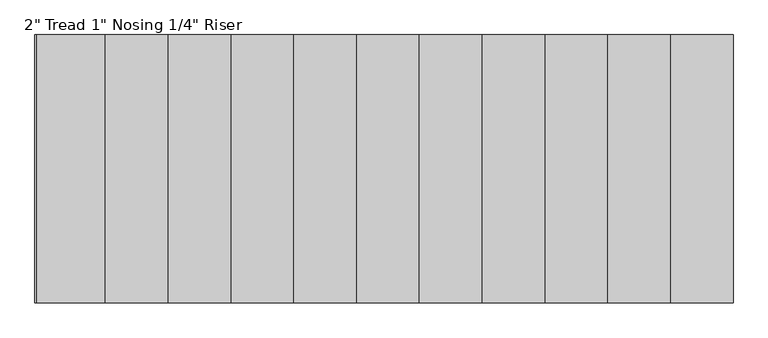
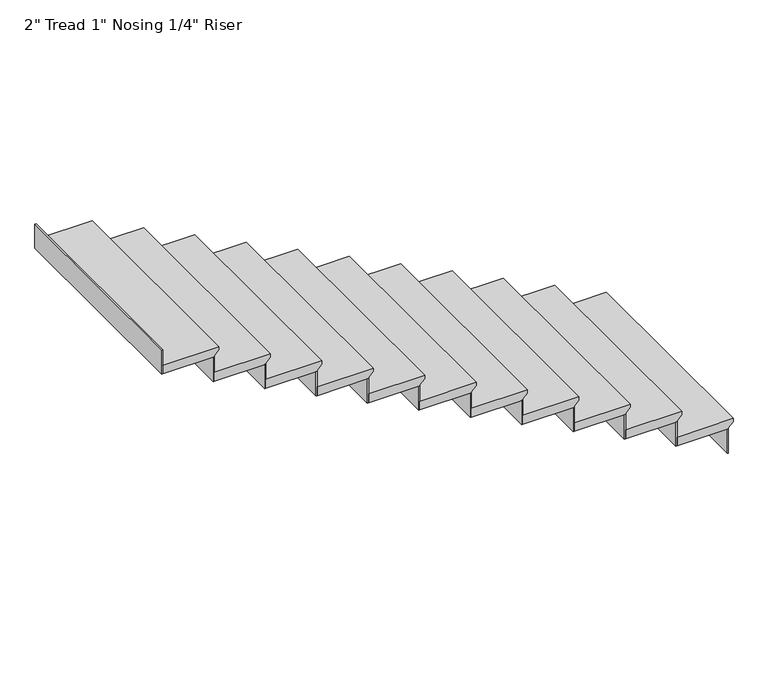
"""IFC4 building model written with IfcOpenShell, lengths in millimetres: stair flight geometry."""

from ifc_helpers import new_model, si_unit, frame, origin, place, context, project, spatial, polyline, outline, extrude, source, transform, mapped, element, save


def stair_flight_7751b166(model_context):
    return source(origin(), model_context, "Body", "SweptSolid", [
        extrude(outline(polyline([(4870.173913, -9934.0183666), (4870.173913, -10238.8183666), (4819.373913, -10238.8183666), (4819.373913, -9959.4183666), (4825.723913, -9959.4183666), (4851.123913, -9934.0183666), (4870.173913, -9934.0183666)])), frame((0.0, 869.1503619, 0.0), z_axis=(0.0, 1.0, 0.0), x_axis=(0.0, 0.0, 1.0)), (0.0, 0.0, 1.0), 1193.8),
        extrude(outline(polyline([(-9965.7683666, 2062.9503619), (-9959.4183666, 2062.9503619), (-9959.4183666, 869.1503619), (-9965.7683666, 869.1503619), (-9965.7683666, 2062.9503619)])), frame((0.0, 0.0, 4680.226087), z_axis=(0.0, 0.0, 1.0), x_axis=(1.0, 0.0, 0.0)), (0.0, 0.0, 1.0), 139.1478261),
        extrude(outline(polyline([(-10245.1683666, 2062.9503619), (-10238.8183666, 2062.9503619), (-10238.8183666, 869.1503619), (-10245.1683666, 869.1503619), (-10245.1683666, 2062.9503619)])), frame((0.0, 0.0, 4819.373913), z_axis=(0.0, 0.0, 1.0), x_axis=(1.0, 0.0, 0.0)), (0.0, 0.0, 1.0), 139.1478261),
        extrude(outline(polyline([(5009.3217391, -10213.4183666), (5009.3217391, -10518.2183666), (4958.5217391, -10518.2183666), (4958.5217391, -10238.8183666), (4964.8717391, -10238.8183666), (4990.2717391, -10213.4183666), (5009.3217391, -10213.4183666)])), frame((0.0, 869.1503619, 0.0), z_axis=(0.0, 1.0, 0.0), x_axis=(0.0, 0.0, 1.0)), (0.0, 0.0, 1.0), 1193.8),
        extrude(outline(polyline([(-10524.5683666, 2062.9503619), (-10518.2183666, 2062.9503619), (-10518.2183666, 869.1503619), (-10524.5683666, 869.1503619), (-10524.5683666, 2062.9503619)])), frame((0.0, 0.0, 4958.5217391), z_axis=(0.0, 0.0, 1.0), x_axis=(1.0, 0.0, 0.0)), (0.0, 0.0, 1.0), 139.1478261),
        extrude(outline(polyline([(5148.4695652, -10492.8183666), (5148.4695652, -10797.6183666), (5097.6695652, -10797.6183666), (5097.6695652, -10518.2183666), (5104.0195652, -10518.2183666), (5129.4195652, -10492.8183666), (5148.4695652, -10492.8183666)])), frame((0.0, 869.1503619, 0.0), z_axis=(0.0, 1.0, 0.0), x_axis=(0.0, 0.0, 1.0)), (0.0, 0.0, 1.0), 1193.8),
        extrude(outline(polyline([(-10803.9683666, 2062.9503619), (-10797.6183666, 2062.9503619), (-10797.6183666, 869.1503619), (-10803.9683666, 869.1503619), (-10803.9683666, 2062.9503619)])), frame((0.0, 0.0, 5097.6695652), z_axis=(0.0, 0.0, 1.0), x_axis=(1.0, 0.0, 0.0)), (0.0, 0.0, 1.0), 139.1478261),
        extrude(outline(polyline([(5287.6173913, -10772.2183666), (5287.6173913, -11077.0183666), (5236.8173913, -11077.0183666), (5236.8173913, -10797.6183666), (5243.1673913, -10797.6183666), (5268.5673913, -10772.2183666), (5287.6173913, -10772.2183666)])), frame((0.0, 869.1503619, 0.0), z_axis=(0.0, 1.0, 0.0), x_axis=(0.0, 0.0, 1.0)), (0.0, 0.0, 1.0), 1193.8),
        extrude(outline(polyline([(-11083.3683666, 2062.9503619), (-11077.0183666, 2062.9503619), (-11077.0183666, 869.1503619), (-11083.3683666, 869.1503619), (-11083.3683666, 2062.9503619)])), frame((0.0, 0.0, 5236.8173913), z_axis=(0.0, 0.0, 1.0), x_axis=(1.0, 0.0, 0.0)), (0.0, 0.0, 1.0), 139.1478261),
        extrude(outline(polyline([(5426.7652174, -11051.6183666), (5426.7652174, -11356.4183666), (5375.9652174, -11356.4183666), (5375.9652174, -11077.0183666), (5382.3152174, -11077.0183666), (5407.7152174, -11051.6183666), (5426.7652174, -11051.6183666)])), frame((0.0, 869.1503619, 0.0), z_axis=(0.0, 1.0, 0.0), x_axis=(0.0, 0.0, 1.0)), (0.0, 0.0, 1.0), 1193.8),
        extrude(outline(polyline([(-11362.7683666, 2062.9503619), (-11356.4183666, 2062.9503619), (-11356.4183666, 869.1503619), (-11362.7683666, 869.1503619), (-11362.7683666, 2062.9503619)])), frame((0.0, 0.0, 5375.9652174), z_axis=(0.0, 0.0, 1.0), x_axis=(1.0, 0.0, 0.0)), (0.0, 0.0, 1.0), 139.1478261),
        extrude(outline(polyline([(5565.9130435, -11331.0183666), (5565.9130435, -11635.8183666), (5515.1130435, -11635.8183666), (5515.1130435, -11356.4183666), (5521.4630435, -11356.4183666), (5546.8630435, -11331.0183666), (5565.9130435, -11331.0183666)])), frame((0.0, 869.1503619, 0.0), z_axis=(0.0, 1.0, 0.0), x_axis=(0.0, 0.0, 1.0)), (0.0, 0.0, 1.0), 1193.8),
        extrude(outline(polyline([(-11642.1683666, 2062.9503619), (-11635.8183666, 2062.9503619), (-11635.8183666, 869.1503619), (-11642.1683666, 869.1503619), (-11642.1683666, 2062.9503619)])), frame((0.0, 0.0, 5515.1130435), z_axis=(0.0, 0.0, 1.0), x_axis=(1.0, 0.0, 0.0)), (0.0, 0.0, 1.0), 139.1478261),
        extrude(outline(polyline([(5705.0608696, -11610.4183666), (5705.0608696, -11915.2183666), (5654.2608696, -11915.2183666), (5654.2608696, -11635.8183666), (5660.6108696, -11635.8183666), (5686.0108696, -11610.4183666), (5705.0608696, -11610.4183666)])), frame((0.0, 869.1503619, 0.0), z_axis=(0.0, 1.0, 0.0), x_axis=(0.0, 0.0, 1.0)), (0.0, 0.0, 1.0), 1193.8),
        extrude(outline(polyline([(-11921.5683666, 2062.9503619), (-11915.2183666, 2062.9503619), (-11915.2183666, 869.1503619), (-11921.5683666, 869.1503619), (-11921.5683666, 2062.9503619)])), frame((0.0, 0.0, 5654.2608696), z_axis=(0.0, 0.0, 1.0), x_axis=(1.0, 0.0, 0.0)), (0.0, 0.0, 1.0), 139.1478261),
        extrude(outline(polyline([(5844.2086957, -11889.8183666), (5844.2086957, -12194.6183666), (5793.4086957, -12194.6183666), (5793.4086957, -11915.2183666), (5799.7586957, -11915.2183666), (5825.1586957, -11889.8183666), (5844.2086957, -11889.8183666)])), frame((0.0, 869.1503619, 0.0), z_axis=(0.0, 1.0, 0.0), x_axis=(0.0, 0.0, 1.0)), (0.0, 0.0, 1.0), 1193.8),
        extrude(outline(polyline([(-12200.9683666, 2062.9503619), (-12194.6183666, 2062.9503619), (-12194.6183666, 869.1503619), (-12200.9683666, 869.1503619), (-12200.9683666, 2062.9503619)])), frame((0.0, 0.0, 5793.4086957), z_axis=(0.0, 0.0, 1.0), x_axis=(1.0, 0.0, 0.0)), (0.0, 0.0, 1.0), 139.1478261),
        extrude(outline(polyline([(5983.3565217, -12169.2183666), (5983.3565217, -12474.0183666), (5932.5565217, -12474.0183666), (5932.5565217, -12194.6183666), (5938.9065217, -12194.6183666), (5964.3065217, -12169.2183666), (5983.3565217, -12169.2183666)])), frame((0.0, 869.1503619, 0.0), z_axis=(0.0, 1.0, 0.0), x_axis=(0.0, 0.0, 1.0)), (0.0, 0.0, 1.0), 1193.8),
        extrude(outline(polyline([(-12480.3683666, 2062.9503619), (-12474.0183666, 2062.9503619), (-12474.0183666, 869.1503619), (-12480.3683666, 869.1503619), (-12480.3683666, 2062.9503619)])), frame((0.0, 0.0, 5932.5565217), z_axis=(0.0, 0.0, 1.0), x_axis=(1.0, 0.0, 0.0)), (0.0, 0.0, 1.0), 139.1478261),
        extrude(outline(polyline([(6122.5043478, -12448.6183666), (6122.5043478, -12753.4183666), (6071.7043478, -12753.4183666), (6071.7043478, -12474.0183666), (6078.0543478, -12474.0183666), (6103.4543478, -12448.6183666), (6122.5043478, -12448.6183666)])), frame((0.0, 869.1503619, 0.0), z_axis=(0.0, 1.0, 0.0), x_axis=(0.0, 0.0, 1.0)), (0.0, 0.0, 1.0), 1193.8),
        extrude(outline(polyline([(-12759.7683666, 2062.9503619), (-12753.4183666, 2062.9503619), (-12753.4183666, 869.1503619), (-12759.7683666, 869.1503619), (-12759.7683666, 2062.9503619)])), frame((0.0, 0.0, 6071.7043478), z_axis=(0.0, 0.0, 1.0), x_axis=(1.0, 0.0, 0.0)), (0.0, 0.0, 1.0), 139.1478261),
        extrude(outline(polyline([(-13039.1683666, 2062.9503619), (-13032.8183666, 2062.9503619), (-13032.8183666, 869.1503619), (-13039.1683666, 869.1503619), (-13039.1683666, 2062.9503619)])), frame((0.0, 0.0, 6210.8521739), z_axis=(0.0, 0.0, 1.0), x_axis=(1.0, 0.0, 0.0)), (0.0, 0.0, 1.0), 139.1478261),
        extrude(outline(polyline([(6261.6521739, -12728.0183666), (6261.6521739, -13032.8183666), (6210.8521739, -13032.8183666), (6210.8521739, -12753.4183666), (6217.2021739, -12753.4183666), (6242.6021739, -12728.0183666), (6261.6521739, -12728.0183666)])), frame((0.0, 869.1503619, 0.0), z_axis=(0.0, 1.0, 0.0), x_axis=(0.0, 0.0, 1.0)), (0.0, 0.0, 1.0), 1193.8),
    ])


if __name__ == "__main__":
    model = new_model("IFC4")
    model_context = context("Model", 3, world=origin())
    ifc_project = project(units=[si_unit("LENGTHUNIT", "METRE", prefix="MILLI")], contexts=[model_context])
    site = spatial("IfcSite", under=ifc_project)
    building = spatial("IfcBuilding", under=site)
    placement = place(None, origin())
    stair_flight_shape = stair_flight_7751b166(model_context)
    element("IfcStairFlight", 1, ObjectType="2\" Tread 1\" Nosing 1/4\" Riser", at=placement, inside=building, context=model_context, shape_type="MappedRepresentation", body=[
        mapped(stair_flight_shape, transform((0.0, 0.0, 0.0), x_axis=(1.0, 0.0, 0.0), y_axis=(0.0, 1.0, 0.0), z_axis=(0.0, 0.0, 1.0))),
    ])
    save(model, "model.ifc")
